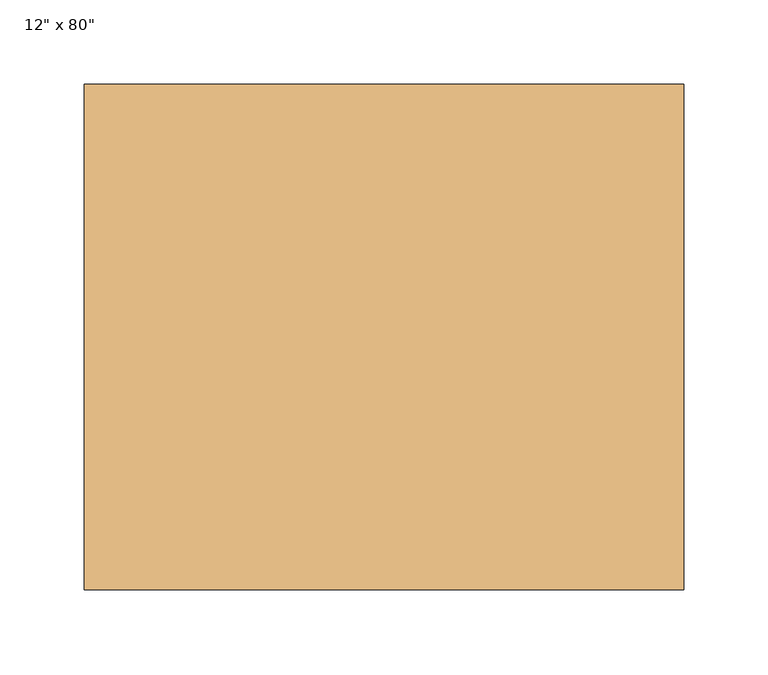
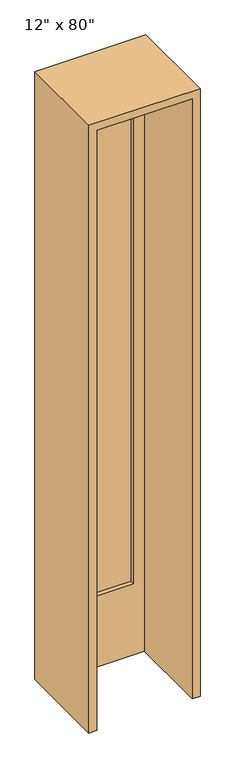
"""IFC4 building model written with IfcOpenShell, lengths in millimetres: door geometry."""

from ifc_helpers import new_model, si_unit, frame, origin, place, context, project, spatial, polyline, outline, extrude, source, transform, mapped, element, save


def door_9a5dd369(model_context):
    return source(origin(), model_context, "Body", "SweptSolid", [
        extrude(outline(polyline([(0.0, 152.4), (0.0, 177.8), (2057.4, 177.8), (2057.4, -177.8), (0.0, -177.8), (0.0, -152.4), (2032.0, -152.4), (2032.0, 152.4), (0.0, 152.4)])), frame((0.0, -153.175, 0.0), z_axis=(0.0, 1.0, 0.0), x_axis=(0.0, 0.0, 1.0)), (0.0, 0.0, 1.0), 300.0),
        extrude(outline(polyline([(2032.0, -152.4), (0.0, -152.4), (0.0, 152.4), (2032.0, 152.4), (2032.0, -152.4)]), holes=[polyline([(241.3, -117.475), (1911.35, -117.475), (1911.35, 117.475), (241.3, 117.475), (241.3, -117.475)])]), frame((0.0, 111.9, 0.0), z_axis=(0.0, 1.0, 0.0), x_axis=(0.0, 0.0, 1.0)), (0.0, 0.0, 1.0), 34.925),
        extrude(outline(polyline([(117.475, 125.87), (-117.475, 125.87), (-117.475, 132.855), (117.475, 132.855), (117.475, 125.87)])), frame((0.0, 0.0, 241.3), z_axis=(0.0, 0.0, 1.0), x_axis=(1.0, 0.0, 0.0)), (0.0, 0.0, 1.0), 1670.05),
    ])


if __name__ == "__main__":
    model = new_model("IFC4")
    model_context = context("Model", 3, world=origin())
    ifc_project = project(units=[si_unit("LENGTHUNIT", "METRE", prefix="MILLI")], contexts=[model_context])
    site = spatial("IfcSite", under=ifc_project)
    building = spatial("IfcBuilding", under=site)
    placement = place(None, origin())
    door_shape = door_9a5dd369(model_context)
    element("IfcDoor", 1, ObjectType="12\" x 80\"", at=placement, inside=building, context=model_context, shape_type="MappedRepresentation", body=[
        mapped(door_shape, transform((0.0, 0.0, 0.0), x_axis=(1.0, 0.0, 0.0), y_axis=(0.0, 1.0, 0.0), z_axis=(0.0, 0.0, 1.0))),
    ])
    save(model, "model.ifc")

# Revit data of these elements
# Type "12\" x 80\""
#   Type Mark = "47"
#   Assembly Code = "B2030100"
#   Analytic Construction = "French door, wood frame with single glass"
#   Top Rail = 120.65 mm
#   Thickness = 34.925 mm
#   Thermal Resistance (R) = 0.188367 (m²·K)/W
#   Stiles = 34.925 mm
#   Rough Width = 355.6 mm
#   Rough Height = 2057.4 mm
#   Height = 2032 mm
#   Width = 304.8 mm
#   Heat Transfer Coefficient (U) = 5.30918 W/(m²·K)
#   Door Offset [instance default] = 0 mm
#   Bottom Rail = 241.3 mm
#   Function = 1
#   Trim Material = Cherry
#   Panel Material = Cherry
#   Glazing = Glass
#   Frame Material = Cherry
#   Visual Light Transmittance = 0
#   Solar Heat Gain Coefficient = 0
#   Wall Closure = (empty or 0)
#   Construction Type = (empty or 0)
# Element 1 (IfcDoor, "12\" x 80\"")
#   Materials on its faces: "Cherry", "Glass"
# Materials
#   "Cherry": class "Wood", colour RGB 226 177 128, transparency 0, Description = "Prunus Serotina", Cost = 0
#   "Glass": class "Glass", colour RGB 0 128 192, transparency 0.9, Description = "Soda Lime Glass", Cost = 0
